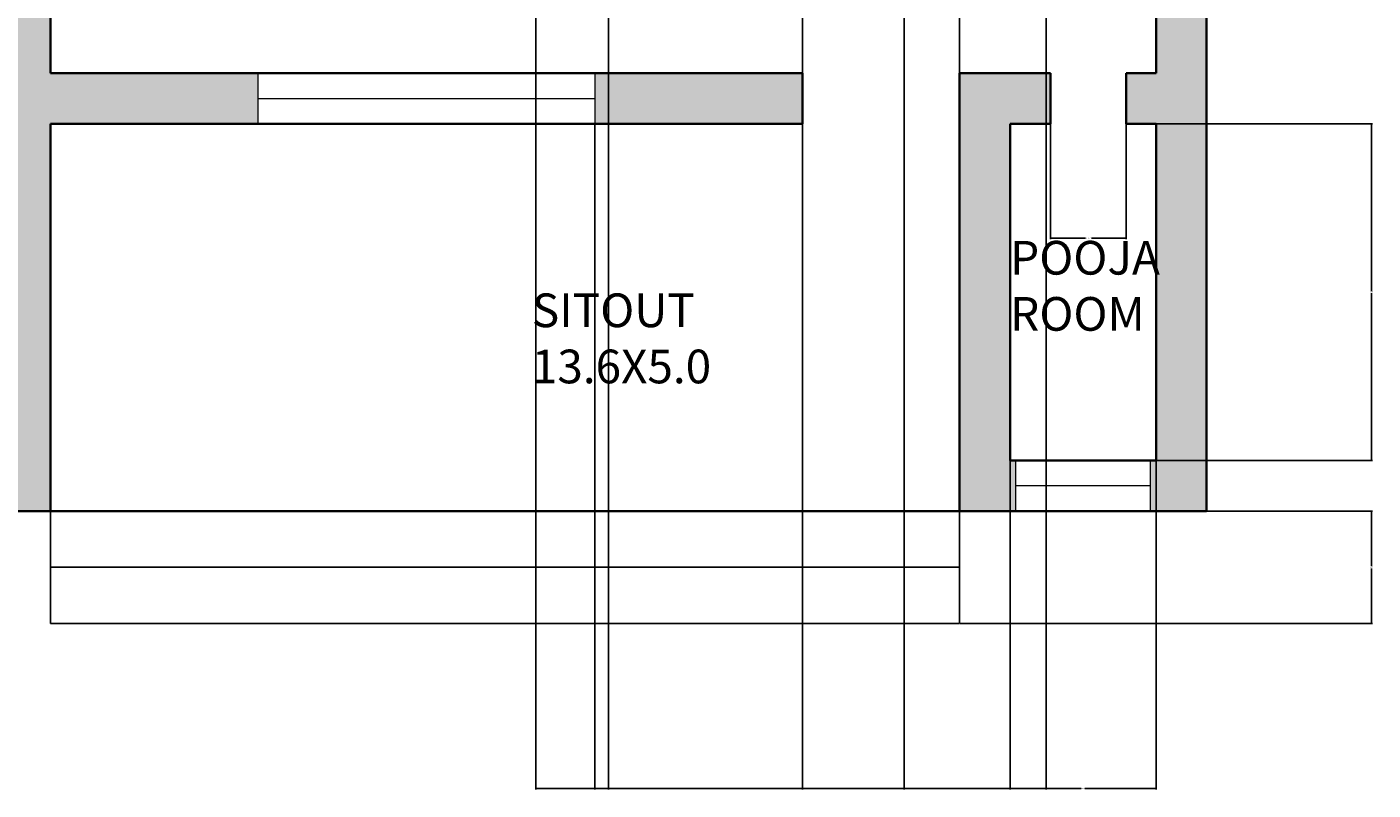
# Model space of a CAD drawing. Units: inches. Extents: x 0 to 423, y -517 to 94.
# Tile 2 of 8: x 182 to 422, y -517 to -382. Entities that reach past the tile are written whole.
import ezdxf

# ---------------------------------------------------------------- set-up
doc = ezdxf.new("R2010")
doc.units = ezdxf.units.IN
doc.header["$MEASUREMENT"] = 0
for name, color, linetype, lineweight in [('A-ANNO-DIMS', 2, 'Continuous', 18), ('A-AREA-IDEN', 7, 'Continuous', 18), ('A-FLOR-STRS', 7, 'Continuous', 25), ('A-GLAZ', 4, 'Continuous', 18), ('A-WALL', 7, 'Continuous', 35)]:
    doc.layers.add(name, color=color, linetype=linetype, lineweight=lineweight)
doc.layers.add('A-WALL-PATT', color=30, linetype='Continuous', lineweight=13, true_color=0xf26722)
doc.styles.get("Standard").update_dxf_attribs({"font": 'arial.ttf'})
doc.dimstyles.get("Standard").update_dxf_attribs({"dimtxt": 0.18, "dimasz": 0.18, "dimexe": 0.18, "dimexo": 0.0625, "dimgap": 0.09, "dimtad": 0, "dimtih": 1, "dimtoh": 1, "dimdec": 0, "dimzin": 0, "dimdsep": 46, "dimlunit": 3, "dimtxsty": 'Standard', "dimcen": 0.09, "dimadec": 0, "dimazin": 0, "dimtfac": 1, "dimtdec": 0, "dimtofl": 0, "dimtmove": 0, "dimatfit": 3, "dimfxl": 1, "dimtolj": 1, "dimtzin": 0, "dimarcsym": 0})

# ---------------------------------------------------------------- blocks, each defined once
blk = doc.blocks.new('WIN-GLAZ-60IN')
for p, q in [((0, 60), (0, 0)), ((4.5, 60), (4.5, 0)), ((9, 0), (9, 60))]:
    blk.add_line(p, q)
blk = doc.blocks.new('WIN-GLAZ-24IN')
for p, q in [((0, 0), (0, 24)), ((4.5, 0), (4.5, 24)), ((9, 24), (9, 0))]:
    blk.add_line(p, q)
blk = doc.blocks.new('*D30')
at = {"layer": 'A-ANNO-DIMS', "color": 0, "lineweight": -2, "transparency": 16777216}
for p, q in [((357.72, -458.83), (357.72, -517.35)), ((383.72, -458.83), (383.72, -517.35)), ((357.9, -517.17), (370.39, -517.17)), ((383.54, -517.17), (371.05, -517.17))]:
    blk.add_line(p, q, dxfattribs=at)
at = {"layer": 'A-ANNO-DIMS', "color": 0, "transparency": 16777216}
for points in [[(357.9, -517.14), (357.9, -517.2), (357.72, -517.17)], [(383.54, -517.14), (383.54, -517.2), (383.72, -517.17)]]:
    blk.add_solid(points, dxfattribs=at)
at = {"layer": 'Defpoints', "color": 0, "transparency": 16777216}
for p in [(357.72, -458.77), (383.72, -458.77), (383.72, -517.17)]:
    blk.add_point(p, dxfattribs=at)
at = {"layer": 'A-ANNO-DIMS', "color": 0, "transparency": 16777216, "insert": (370.72, -517.17), "char_height": 0.18, "attachment_point": 5}
blk.add_mtext('\\A1;2\'-2"', dxfattribs=at)
blk = doc.blocks.new('*D31')
at = {"layer": 'A-ANNO-DIMS', "color": 0, "lineweight": -2, "transparency": 16777216}
for p, q in [((383.79, -398.77), (422.3, -398.77)), ((422.12, -398.95), (422.12, -428.58)), ((422.12, -458.59), (422.12, -428.95)), ((383.79, -458.77), (422.3, -458.77))]:
    blk.add_line(p, q, dxfattribs=at)
at = {"layer": 'A-ANNO-DIMS', "color": 0, "transparency": 16777216}
for points in [[(422.09, -398.95), (422.15, -398.95), (422.12, -398.77)], [(422.09, -458.59), (422.15, -458.59), (422.12, -458.77)]]:
    blk.add_solid(points, dxfattribs=at)
at = {"layer": 'Defpoints', "color": 0, "transparency": 16777216}
for p in [(383.72, -398.77), (422.12, -398.77), (383.72, -458.77)]:
    blk.add_point(p, dxfattribs=at)
at = {"layer": 'A-ANNO-DIMS', "color": 0, "transparency": 16777216, "insert": (422.12, -428.77), "char_height": 0.18, "attachment_point": 5}
blk.add_mtext('\\A1;5\'-0"', dxfattribs=at)
blk = doc.blocks.new('*D32')
at = {"layer": 'A-ANNO-DIMS', "color": 0, "lineweight": -2, "transparency": 16777216}
for p, q in [((348.79, -467.77), (422.3, -467.77)), ((422.12, -467.95), (422.12, -477.58)), ((422.12, -487.59), (422.12, -477.95)), ((348.79, -487.77), (422.3, -487.77))]:
    blk.add_line(p, q, dxfattribs=at)
at = {"layer": 'A-ANNO-DIMS', "color": 0, "transparency": 16777216}
for points in [[(422.09, -467.95), (422.15, -467.95), (422.12, -467.77)], [(422.09, -487.59), (422.15, -487.59), (422.12, -487.77)]]:
    blk.add_solid(points, dxfattribs=at)
at = {"layer": 'Defpoints', "color": 0, "transparency": 16777216}
for p in [(348.72, -467.77), (422.12, -467.77), (348.72, -487.77)]:
    blk.add_point(p, dxfattribs=at)
at = {"layer": 'A-ANNO-DIMS', "color": 0, "transparency": 16777216, "insert": (422.12, -477.77), "char_height": 0.18, "attachment_point": 5}
blk.add_mtext('\\A1;1\'-8"', dxfattribs=at)
blk = doc.blocks.new('*D35')
at = {"layer": 'A-ANNO-DIMS', "color": 0, "lineweight": -2, "transparency": 16777216}
for p, q in [((320.72, -389.7), (320.72, 45.81)), ((320.9, 45.63), (334.39, 45.63)), ((348.54, 45.63), (335.05, 45.63)), ((348.72, -389.7), (348.72, 45.81))]:
    blk.add_line(p, q, dxfattribs=at)
at = {"layer": 'A-ANNO-DIMS', "color": 0, "transparency": 16777216}
for points in [[(320.9, 45.66), (320.9, 45.6), (320.72, 45.63)], [(348.54, 45.66), (348.54, 45.6), (348.72, 45.63)]]:
    blk.add_solid(points, dxfattribs=at)
at = {"layer": 'Defpoints', "color": 0, "transparency": 16777216}
for p in [(348.72, 45.63), (320.72, -389.77), (348.72, -389.77)]:
    blk.add_point(p, dxfattribs=at)
at = {"layer": 'A-ANNO-DIMS', "color": 0, "transparency": 16777216, "insert": (334.72, 45.63), "char_height": 0.18, "attachment_point": 5}
blk.add_mtext('\\A1;2\'-4"', dxfattribs=at)
blk = doc.blocks.new('*D36')
at = {"layer": 'A-ANNO-DIMS', "color": 0, "lineweight": -2, "transparency": 16777216}
for p, q in [((283.72, -398.83), (283.72, -517.35)), ((320.72, -398.83), (320.72, -517.35)), ((283.9, -517.17), (301.89, -517.17)), ((320.54, -517.17), (302.55, -517.17))]:
    blk.add_line(p, q, dxfattribs=at)
at = {"layer": 'A-ANNO-DIMS', "color": 0, "transparency": 16777216}
for points in [[(283.9, -517.14), (283.9, -517.2), (283.72, -517.17)], [(320.54, -517.14), (320.54, -517.2), (320.72, -517.17)]]:
    blk.add_solid(points, dxfattribs=at)
at = {"layer": 'Defpoints', "color": 0, "transparency": 16777216}
for p in [(283.72, -398.77), (320.72, -398.77), (320.72, -517.17)]:
    blk.add_point(p, dxfattribs=at)
at = {"layer": 'A-ANNO-DIMS', "color": 0, "transparency": 16777216, "insert": (302.22, -517.17), "char_height": 0.18, "attachment_point": 5}
blk.add_mtext('\\A1;3\'-1"', dxfattribs=at)
blk = doc.blocks.new('*D37')
at = {"layer": 'A-ANNO-DIMS', "color": 0, "lineweight": -2, "transparency": 16777216}
for p, q in [((364.92, -389.83), (364.92, -419.35)), ((378.42, -389.83), (378.42, -419.35)), ((365.1, -419.17), (371.14, -419.17)), ((378.24, -419.17), (372.2, -419.17))]:
    blk.add_line(p, q, dxfattribs=at)
at = {"layer": 'A-ANNO-DIMS', "color": 0, "transparency": 16777216}
for points in [[(365.1, -419.14), (365.1, -419.2), (364.92, -419.17)], [(378.24, -419.14), (378.24, -419.2), (378.42, -419.17)]]:
    blk.add_solid(points, dxfattribs=at)
at = {"layer": 'Defpoints', "color": 0, "transparency": 16777216}
for p in [(364.92, -389.77), (378.42, -389.77), (364.92, -419.17)]:
    blk.add_point(p, dxfattribs=at)
at = {"layer": 'A-ANNO-DIMS', "color": 0, "transparency": 16777216, "insert": (371.67, -419.17), "char_height": 0.18, "attachment_point": 5}
blk.add_mtext('\\A1;1\'-1 1/2"', dxfattribs=at)
blk = doc.blocks.new('*D50')
at = {"layer": 'A-ANNO-DIMS', "color": 0, "lineweight": -2, "transparency": 16777216}
for p, q in [((273.19, -103.61), (273.19, -517.35)), ((364.14, -103.61), (364.14, -517.35)), ((273.37, -517.17), (318.34, -517.17)), ((363.96, -517.17), (318.99, -517.17))]:
    blk.add_line(p, q, dxfattribs=at)
at = {"layer": 'A-ANNO-DIMS', "color": 0, "transparency": 16777216}
for points in [[(273.37, -517.14), (273.37, -517.2), (273.19, -517.17)], [(363.96, -517.14), (363.96, -517.2), (364.14, -517.17)]]:
    blk.add_solid(points, dxfattribs=at)
at = {"layer": 'Defpoints', "color": 0, "transparency": 16777216}
for p in [(273.19, -103.55), (364.14, -103.55), (364.14, -517.17)]:
    blk.add_point(p, dxfattribs=at)
at = {"layer": 'A-ANNO-DIMS', "color": 0, "transparency": 16777216, "insert": (318.66, -517.17), "char_height": 0.18, "attachment_point": 5}
blk.add_mtext('\\A1;7\'-7"', dxfattribs=at)
blk = doc.blocks.new('*D51')
at = {"layer": 'A-ANNO-DIMS', "color": 0, "lineweight": -2, "transparency": 16777216}
for p, q in [((286.14, -253.61), (286.14, -517.35)), ((338.82, -253.61), (338.82, -517.35)), ((286.32, -517.17), (311.93, -517.17)), ((338.64, -517.17), (313.02, -517.17))]:
    blk.add_line(p, q, dxfattribs=at)
at = {"layer": 'A-ANNO-DIMS', "color": 0, "transparency": 16777216}
for points in [[(286.32, -517.14), (286.32, -517.2), (286.14, -517.17)], [(338.64, -517.14), (338.64, -517.2), (338.82, -517.17)]]:
    blk.add_solid(points, dxfattribs=at)
at = {"layer": 'Defpoints', "color": 0, "transparency": 16777216}
for p in [(286.14, -253.55), (338.82, -253.55), (338.82, -517.17)]:
    blk.add_point(p, dxfattribs=at)
at = {"layer": 'A-ANNO-DIMS', "color": 0, "transparency": 16777216, "insert": (312.48, -517.17), "char_height": 0.18, "attachment_point": 5}
blk.add_mtext('\\A1;4\'-4 1/2"', dxfattribs=at)

msp = doc.modelspace()

# ---------------------------------------------------------------- hatches: boundary and pattern name
at = {"layer": 'A-WALL-PATT'}
h = msp.add_hatch(color=256, dxfattribs=at)
h.dxf.hatch_style = 1
h.paths.add_polyline_path([(201.52, 16.23), (138.22, 16.23), (138.22, 7.23), (177.72, 7.23), (177.72, -138.77), (186.72, -138.77), (186.72, -92.77), (251.72, -92.77), (251.72, -22.53), (242.72, -22.53), (242.72, -83.77), (186.72, -83.77), (186.72, 7.23), (201.52, 7.23)])
h.paths.add_polyline_path([(78.22, 16.23), (29.72, 16.23), (29.72, -31.27), (38.72, -31.27), (38.72, 7.23), (78.22, 7.23)])
h.paths.add_polyline_path([(275.31, 16.23), (225.52, 16.23), (225.52, 7.23), (275.31, 7.23)])
h.paths.add_polyline_path([(392.72, 16.23), (335.31, 16.23), (335.31, 7.23), (383.72, 7.23), (383.72, -31.27), (392.72, -31.27)])
h.paths.add_polyline_path([(143.33, -129.77), (38.72, -129.77), (38.72, -91.27), (29.72, -91.27), (29.72, -157.27), (38.72, -157.27), (38.72, -138.77), (143.33, -138.77)])
h.paths.add_polyline_path([(186.72, -199.77), (38.72, -199.77), (38.72, -181.27), (29.72, -181.27), (29.72, -239.27), (38.72, -239.27), (38.72, -208.77), (177.72, -208.77), (177.72, -237.07), (186.72, -237.07)])
h.paths.add_polyline_path([(111.72, -161.55), (102.72, -161.55), (102.72, -199.77), (111.72, -199.77)])
h.paths.add_polyline_path([(392.72, -91.27), (383.72, -91.27), (383.72, -129.77), (242.72, -129.77), (242.72, -138.77), (383.72, -138.77), (383.72, -169.77), (392.72, -169.77)])
h.paths.add_polyline_path([(392.72, -229.77), (383.72, -229.77), (383.72, -262.77), (251.72, -262.77), (251.72, -177.14), (242.72, -177.14), (242.72, -271.77), (383.72, -271.77), (383.72, -300.77), (392.72, -300.77)])
h.paths.add_polyline_path([(392.72, -360.77), (383.72, -360.77), (383.72, -389.77), (378.42, -389.77), (378.42, -398.77), (383.72, -398.77), (383.72, -458.77), (382.72, -458.77), (382.72, -467.77), (392.72, -467.77)])
h.paths.add_polyline_path([(364.92, -389.77), (348.72, -389.77), (348.72, -467.77), (358.72, -467.77), (358.72, -458.77), (357.72, -458.77), (357.72, -398.77), (364.92, -398.77)])
h.paths.add_polyline_path([(320.72, -389.77), (283.72, -389.77), (283.72, -398.77), (320.72, -398.77)])
h.paths.add_polyline_path([(223.72, -389.77), (186.72, -389.77), (186.72, -270.38), (177.72, -270.38), (177.72, -458.77), (138.22, -458.77), (138.22, -467.77), (186.72, -467.77), (186.72, -398.77), (223.72, -398.77)])
h.paths.add_polyline_path([(143.29, -329.77), (38.72, -329.77), (38.72, -299.27), (29.72, -299.27), (29.72, -338.77), (143.29, -338.77)])
h.paths.add_polyline_path([(38.72, -374.71), (29.72, -374.71), (29.72, -398.74), (38.72, -398.74)])
h.paths.add_polyline_path([(78.22, -458.77), (38.72, -458.77), (38.72, -434.74), (29.72, -434.74), (29.72, -467.77), (78.22, -467.77)])
h.paths.add_polyline_path([(279.99, -158.17), (326.6, -158.17), (326.6, -135.78), (279.99, -135.78)], flags=25)
h.paths.add_polyline_path([(355.56, -439.13), (387, -439.13), (387, -416.66), (355.56, -416.66)], flags=9)

# ---------------------------------------------------------------- linework, layer by layer
at = {"layer": 'A-FLOR-STRS'}
for p, q in [((186.72, -467.77), (186.72, -477.77)), ((348.72, -487.77), (348.72, -467.77)), ((186.72, -477.77), (186.72, -487.77)), ((186.72, -477.77), (348.72, -477.77)), ((186.72, -487.77), (348.72, -487.77))]:
    msp.add_line(p, q, dxfattribs=at)
at = {"layer": 'A-GLAZ'}
for p, q in [((223.72, -398.77), (223.72, -389.77)), ((283.72, -389.77), (283.72, -398.77)), ((358.72, -467.77), (358.72, -458.77)), ((382.72, -467.77), (382.72, -458.77))]:
    msp.add_line(p, q, dxfattribs=at)
at = {"layer": 'A-WALL'}
for p, q in [((392.72, 16.23), (392.72, -467.77)), ((186.72, -270.38), (186.72, -389.77)), ((383.72, -271.77), (383.72, -389.77)), ((186.72, -389.77), (320.72, -389.77)), ((320.72, -389.77), (320.72, -398.77)), ((348.72, -389.77), (348.72, -467.77)), ((348.72, -389.77), (364.92, -389.77)), ((364.92, -389.77), (364.92, -398.77)), ((378.42, -389.77), (378.42, -398.77)), ((378.42, -389.77), (383.72, -389.77)), ((186.72, -398.77), (320.72, -398.77)), ((186.72, -398.77), (186.72, -467.77)), ((357.72, -398.77), (357.72, -458.77)), ((357.72, -398.77), (364.92, -398.77)), ((378.42, -398.77), (383.72, -398.77)), ((383.72, -398.77), (383.72, -458.77)), ((357.72, -458.77), (383.72, -458.77)), ((29.72, -467.77), (392.72, -467.77))]:
    msp.add_line(p, q, dxfattribs=at)

# ---------------------------------------------------------------- block references
at = {"layer": 'A-GLAZ'}
for name, p, rotation in [('WIN-GLAZ-60IN', (283.72, -398.76), 90), ('WIN-GLAZ-24IN', (382.72, -467.76), 89.9999999999998)]:
    msp.add_blockref(name, p, dxfattribs=dict(at, rotation=rotation))

# ---------------------------------------------------------------- texts
at = {"layer": 'A-AREA-IDEN', "char_height": 6, "attachment_point": 1}
for s, insert in [('POOJA\\PROOM', (357.72, -419.64)), ('SITOUT\\P13.6X5.0', (272.48, -429))]:
    msp.add_mtext(s, dxfattribs=dict(at, insert=insert))

# ---------------------------------------------------------------- dimensions: what is measured, and where the dimension line sits
at = {"layer": 'A-ANNO-DIMS'}
for base, p1, p2, picture, middle in [((348.72, 45.63), (320.72, -389.77), (348.72, -389.77), '*D35', (334.72, 45.63)), ((364.1422, -517.1651), (273.186, -103.5478), (364.1422, -103.5478), '*D50', (318.6641, -517.1651)), ((338.82, -517.17), (286.14, -253.55), (338.82, -253.55), '*D51', (312.48, -517.17)), ((320.72, -517.17), (283.72, -398.77), (320.72, -398.77), '*D36', (302.22, -517.17)), ((383.72, -517.17), (357.72, -458.77), (383.72, -458.77), '*D30', (370.72, -517.17))]:
    dim = msp.add_linear_dim(base=base, p1=p1, p2=p2, dimstyle='Standard', override={"dimdec": 1, "dimlfac": 1, "dimrnd": 0, "dimzin": 1, "dimdsep": 46, "dimlunit": 4, "dimfrac": 2}, dxfattribs=at)
    dim.commit()
    dim.dimension.update_dxf_attribs({"geometry": picture, "text_midpoint": middle})
for base, p1, p2, angle, picture, middle in [((364.92, -419.17), (378.42, -389.77), (364.92, -389.77), 180, '*D37', (371.67, -419.17)), ((422.12, -398.77), (383.72, -458.77), (383.72, -398.77), 90, '*D31', (422.12, -428.77)), ((422.12, -467.77), (348.72, -487.77), (348.72, -467.77), 90, '*D32', (422.12, -477.77))]:
    dim = msp.add_linear_dim(base=base, p1=p1, p2=p2, angle=angle, dimstyle='Standard', override={"dimdec": 1, "dimlfac": 1, "dimrnd": 0, "dimzin": 1, "dimdsep": 46, "dimlunit": 4, "dimfrac": 2}, dxfattribs=at)
    dim.commit()
    dim.dimension.update_dxf_attribs({"geometry": picture, "text_midpoint": middle})

doc.saveas('drawing.dxf')
